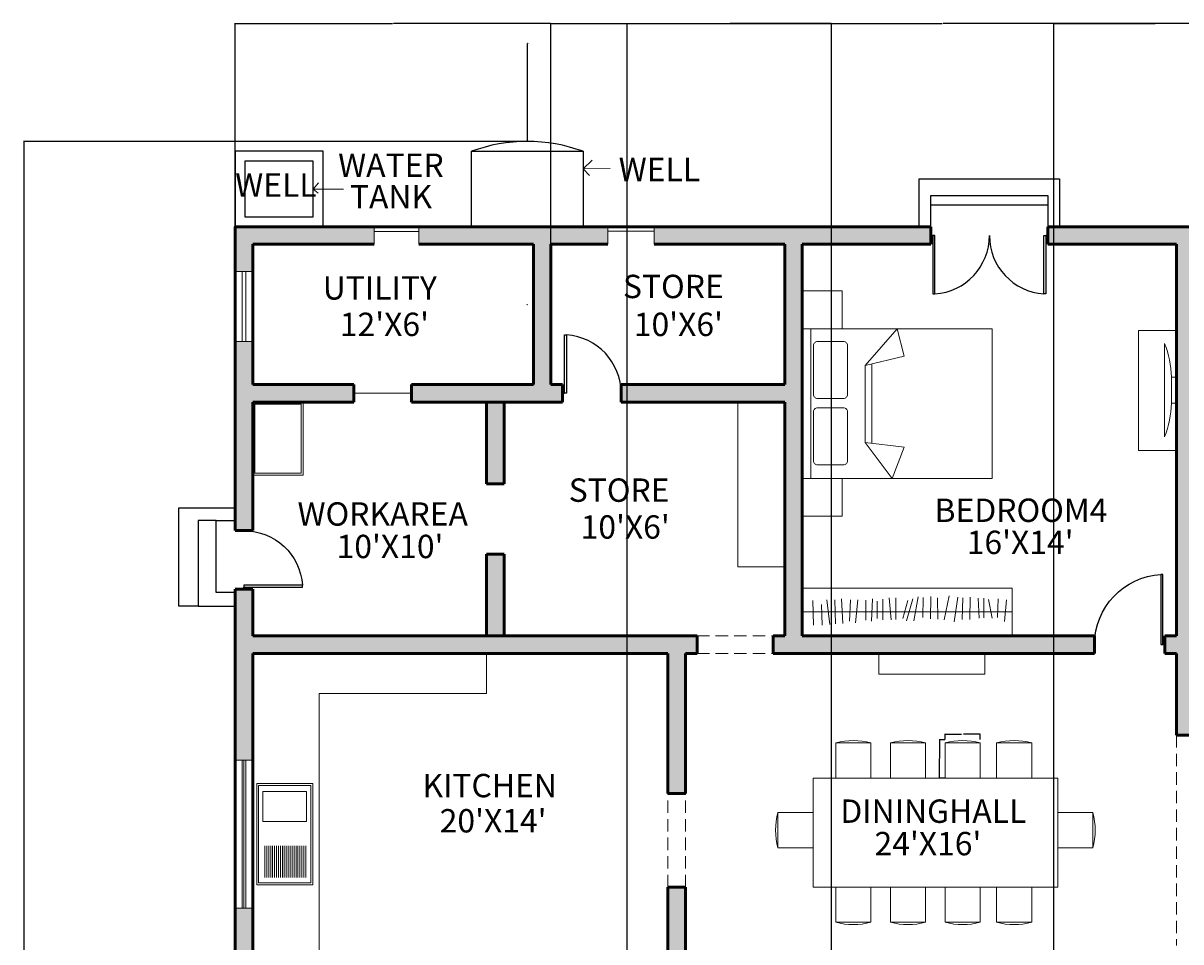
# Model space of a CAD drawing. Units: inches. Extents: x 2743 to 3669, y 1014 to 2282.
# Tile 4 of 5: x 2743 to 3337, y 1810 to 2282. Entities that reach past the tile are written whole.
import ezdxf

# ---------------------------------------------------------------- set-up
doc = ezdxf.new("R2010")
doc.units = ezdxf.units.IN
doc.linetypes.add('DASHED2', pattern=[9.525, 6.35, -3.175])
for name, color, linetype, lineweight in [('A-ANNO-DIMS', 2, 'Continuous', 18), ('A-ANNO-SYMB', 7, 'Continuous', 18), ('A-ANNO-TEXT', 4, 'Continuous', 18), ('A-AREA-IDEN', 4, 'Continuous', 18), ('A-DOOR', 211, 'Continuous', 25), ('A-EQPM', 51, 'Continuous', 18), ('A-FLOR-CASE', 51, 'Continuous', 18), ('A-FLOR-FIXT-PATT', 8, 'Continuous', 13), ('A-FLOR-STRS', 7, 'Continuous', 25), ('A-FURN', 111, 'Continuous', 18), ('A-GLAZ', 40, 'Continuous', 20), ('A-WALL', 7, 'Continuous', 50), ('A-WALL-OVHD', 8, 'DASHED2', 18), ('P-EQPM', 4, 'Continuous', 25)]:
    doc.layers.add(name, color=color, linetype=linetype, lineweight=lineweight)
doc.layers.add('A-FLOR-FIXT', color=11, linetype='Continuous', lineweight=18, true_color=0xee778f)
doc.layers.add('A-WALL-PATT', color=47, linetype='Continuous', lineweight=13, true_color=0x726c55)
doc.styles.get("Standard").update_dxf_attribs({"font": 'arial.ttf'})
doc.dimstyles.get("Standard").update_dxf_attribs({"dimtxt": 0.18, "dimasz": 0.18, "dimexe": 0.18, "dimexo": 0.0625, "dimgap": 0.09, "dimtad": 0, "dimtih": 1, "dimtoh": 1, "dimdec": 4, "dimzin": 0, "dimdsep": 46, "dimtxsty": 'Standard', "dimcen": 0.09, "dimadec": 0, "dimazin": 0, "dimtfac": 1, "dimtdec": 4, "dimtofl": 0, "dimtmove": 0, "dimatfit": 3, "dimfxl": 1, "dimtolj": 1, "dimtzin": 0, "dimarcsym": 0})

# ---------------------------------------------------------------- blocks, each defined once
blk = doc.blocks.new('DOOR-PAIR-60IN')
for p, q in [((0, 30), (1, 30)), ((1, 30), (1, 0)), ((2, 30), (1, 30)), ((2, 0), (2, 30)), ((58, 0), (58, 30)), ((58, 30), (59, 30)), ((60, 30), (59, 30)), ((59, 30), (59, 0)), ((1, 0), (2, 0)), ((59, 0), (58, 0))]:
    blk.add_line(p, q)
for centre, start, end in [((0, 29.93), 273.82241, 0.12746), ((60, 29.93), 179.99998, 266.1773)]:
    blk.add_arc(centre, 30, start, end)
blk = doc.blocks.new('DOOR-SINGLE-30IN')
for p, q in [((1, 0), (1, 30)), ((1, 30), (2, 30)), ((2, 30), (2, 0)), ((0, 0), (1, 0)), ((2, 0), (1, 0))]:
    blk.add_line(p, q)
blk.add_arc((0, 0.07), 30, 359.87254, 86.17759)
blk = doc.blocks.new('DOOR-SINGLE-36IN')
for p, q in [((1, 0), (1, 36)), ((1, 36), (2, 36)), ((2, 36), (2, 0)), ((0, 0), (1, 0)), ((2, 0), (1, 0))]:
    blk.add_line(p, q)
blk.add_arc((0, 0.06), 36, 359.91152, 86.81533)
blk = doc.blocks.new('WINDOW-36IN')
for p, q in [((9, 36), (0, 36)), ((3.5, 36), (3.5, 0)), ((5.5, 36), (5.5, 0)), ((9, 0), (0, 0))]:
    blk.add_line(p, q)
blk = doc.blocks.new('BED-DOUBLE')
for p, q in [((4.31, 76.75), (4.31, 0)), ((32.31, 57.96), (48.69, 76.75)), ((48.69, 76.75), (52.23, 62.72)), ((52.23, 62.72), (32.31, 57.96)), ((32.31, 18.34), (32.31, 57.96)), ((35.7, 17.95), (35.72, 58.78)), ((46.06, 0), (32.31, 18.34)), ((52.23, 16.05), (32.31, 18.34)), ((46.06, 0), (52.23, 16.05))]:
    blk.add_line(p, q)
blk.add_lwpolyline([(0, 76.75), (97.38, 76.75), (97.38, 0), (0, 0)], close=True)
for points in [[(7.76, 70.21), (21.16, 70.21, -0.414214), (23.16, 68.21), (23.16, 43, -0.414214), (21.16, 41), (7.76, 41, -0.414214), (5.76, 43), (5.76, 68.21, -0.414214)], [(7.76, 36.18), (21.16, 36.18, -0.414214), (23.16, 34.18), (23.16, 8.97, -0.414214), (21.16, 6.97), (7.76, 6.97, -0.414214), (5.76, 8.97), (5.76, 34.18, -0.414214)]]:
    blk.add_lwpolyline(points, format="xyb", close=True)
blk = doc.blocks.new('NIGHTSTAND')
blk.add_lwpolyline([(0, 0), (20.5, 0), (20.5, 19.45), (0, 19.45)], close=True)
blk = doc.blocks.new('CHAIR-DINING')
for p, q in [((0, 0), (0, 18)), ((0, 18), (18, 18)), ((18, 18), (18, 0))]:
    blk.add_line(p, q)
blk.add_arc((9, -14.1), 33.34, 74.33691, 105.66309)
blk = doc.blocks.new('*D22')
at = {"layer": 'A-ANNO-DIMS', "color": 0, "lineweight": -2, "transparency": 16777216}
for p, q in [((3216, 1913.74), (3212.93, 1913.74)), ((3213.11, 1913.56), (3213.11, 1904.1)), ((3213.11, 1894.27), (3213.11, 1903.73)), ((3216, 1894.09), (3212.93, 1894.09))]:
    blk.add_line(p, q, dxfattribs=at)
at = {"layer": 'A-ANNO-DIMS', "color": 0, "transparency": 16777216}
for points in [[(3213.08, 1913.56), (3213.14, 1913.56), (3213.11, 1913.74)], [(3213.08, 1894.27), (3213.14, 1894.27), (3213.11, 1894.09)]]:
    blk.add_solid(points, dxfattribs=at)
at = {"layer": 'Defpoints', "color": 0, "transparency": 16777216}
for p in [(3213.11, 1913.74), (3216.06, 1913.74), (3216.06, 1894.09)]:
    blk.add_point(p, dxfattribs=at)
at = {"layer": 'A-ANNO-DIMS', "color": 0, "transparency": 16777216, "insert": (3213.11, 1903.92), "char_height": 0.18, "attachment_point": 5}
blk.add_mtext('\\A1;CHAIR 20 TYP.', dxfattribs=at)
blk = doc.blocks.new('*D23')
at = {"layer": 'A-ANNO-DIMS', "color": 0, "lineweight": -2, "transparency": 16777216}
for p, q in [((3216.06, 1913.8), (3216.06, 1916.87)), ((3216.24, 1916.69), (3224.54, 1916.69)), ((3233.88, 1916.69), (3225.58, 1916.69)), ((3234.06, 1913.8), (3234.06, 1916.87))]:
    blk.add_line(p, q, dxfattribs=at)
at = {"layer": 'A-ANNO-DIMS', "color": 0, "transparency": 16777216}
for points in [[(3216.24, 1916.72), (3216.24, 1916.66), (3216.06, 1916.69)], [(3233.88, 1916.72), (3233.88, 1916.66), (3234.06, 1916.69)]]:
    blk.add_solid(points, dxfattribs=at)
at = {"layer": 'Defpoints', "color": 0, "transparency": 16777216}
for p in [(3216.06, 1913.74), (3234.06, 1916.69), (3234.06, 1913.74)]:
    blk.add_point(p, dxfattribs=at)
at = {"layer": 'A-ANNO-DIMS', "color": 0, "transparency": 16777216, "insert": (3225.06, 1916.69), "char_height": 0.18, "attachment_point": 5}
blk.add_mtext('\\A1;18 TYP.', dxfattribs=at)
blk = doc.blocks.new('*D62')
at = {"layer": 'A-ANNO-DIMS', "color": 0, "lineweight": -2, "transparency": 16777216}
for p, q in [((3608.38, 1899.55), (3608.38, 1014.41)), ((2803.91, 1765.52), (2803.91, 1014.41)), ((2804.09, 1014.59), (3205.75, 1014.59)), ((3608.2, 1014.59), (3206.54, 1014.59))]:
    blk.add_line(p, q, dxfattribs=at)
at = {"layer": 'A-ANNO-DIMS', "color": 0, "transparency": 16777216}
for points in [[(2804.09, 1014.62), (2804.09, 1014.56), (2803.91, 1014.59)], [(3608.2, 1014.62), (3608.2, 1014.56), (3608.38, 1014.59)]]:
    blk.add_solid(points, dxfattribs=at)
at = {"layer": 'Defpoints', "color": 0, "transparency": 16777216}
for p in [(3608.38, 1899.61), (2803.91, 1765.58), (3608.38, 1014.59)]:
    blk.add_point(p, dxfattribs=at)
at = {"layer": 'A-ANNO-DIMS', "color": 0, "transparency": 16777216, "insert": (3206.15, 1014.59), "char_height": 0.18, "attachment_point": 5}
blk.add_mtext('\\A1;804.5', dxfattribs=at)
blk = doc.blocks.new('*D63')
at = {"layer": 'A-ANNO-DIMS', "color": 0, "lineweight": -2, "transparency": 16777216}
for p, q in [((3001.57, 2220.87), (2743.18, 2220.87)), ((2743.36, 2220.69), (2743.36, 1648.19)), ((2743.36, 1075.32), (2743.36, 1647.82)), ((3214.73, 1075.14), (2743.18, 1075.14))]:
    blk.add_line(p, q, dxfattribs=at)
at = {"layer": 'A-ANNO-DIMS', "color": 0, "transparency": 16777216}
for points in [[(2743.33, 2220.69), (2743.39, 2220.69), (2743.36, 2220.87)], [(2743.33, 1075.32), (2743.39, 1075.32), (2743.36, 1075.14)]]:
    blk.add_solid(points, dxfattribs=at)
at = {"layer": 'Defpoints', "color": 0, "transparency": 16777216}
for p in [(2743.36, 2220.87), (3001.63, 2220.87), (3214.8, 1075.14)]:
    blk.add_point(p, dxfattribs=at)
at = {"layer": 'A-ANNO-DIMS', "color": 0, "transparency": 16777216, "insert": (2743.36, 1648.01), "char_height": 0.18, "attachment_point": 5}
blk.add_mtext('\\A1;1145.7', dxfattribs=at)
blk = doc.blocks.new('*D64')
at = {"layer": 'A-ANNO-DIMS', "color": 0, "lineweight": -2, "transparency": 16777216}
for p, q in [((2851.8, 2177.16), (2851.8, 2281.6)), ((2851.98, 2281.42), (2932.52, 2281.42)), ((3013.62, 2281.42), (2933.08, 2281.42)), ((3013.8, 2168.16), (3013.8, 2281.6))]:
    blk.add_line(p, q, dxfattribs=at)
at = {"layer": 'A-ANNO-DIMS', "color": 0, "transparency": 16777216}
for points in [[(2851.98, 2281.45), (2851.98, 2281.39), (2851.8, 2281.42)], [(3013.62, 2281.45), (3013.62, 2281.39), (3013.8, 2281.42)]]:
    blk.add_solid(points, dxfattribs=at)
at = {"layer": 'Defpoints', "color": 0, "transparency": 16777216}
for p in [(3013.8, 2281.42), (2851.8, 2177.09), (3013.8, 2168.09)]:
    blk.add_point(p, dxfattribs=at)
at = {"layer": 'A-ANNO-DIMS', "color": 0, "transparency": 16777216, "insert": (2932.8, 2281.42), "char_height": 0.18, "attachment_point": 5}
blk.add_mtext('\\A1;162', dxfattribs=at)
blk = doc.blocks.new('*D65')
at = {"layer": 'A-ANNO-DIMS', "color": 0, "lineweight": -2, "transparency": 16777216}
for p, q in [((3013.8, 2168.16), (3013.8, 2281.6)), ((3013.98, 2281.42), (3214.5, 2281.42)), ((3415.62, 2281.42), (3215.09, 2281.42)), ((3415.8, 2168.16), (3415.8, 2281.6))]:
    blk.add_line(p, q, dxfattribs=at)
at = {"layer": 'A-ANNO-DIMS', "color": 0, "transparency": 16777216}
for points in [[(3013.98, 2281.45), (3013.98, 2281.39), (3013.8, 2281.42)], [(3415.62, 2281.45), (3415.62, 2281.39), (3415.8, 2281.42)]]:
    blk.add_solid(points, dxfattribs=at)
at = {"layer": 'Defpoints', "color": 0, "transparency": 16777216}
for p in [(3415.8, 2281.42), (3013.8, 2168.09), (3415.8, 2168.09)]:
    blk.add_point(p, dxfattribs=at)
at = {"layer": 'A-ANNO-DIMS', "color": 0, "transparency": 16777216, "insert": (3214.8, 2281.42), "char_height": 0.18, "attachment_point": 5}
blk.add_mtext('\\A1;402', dxfattribs=at)
blk = doc.blocks.new('*D76')
at = {"layer": 'A-ANNO-DIMS', "color": 0, "lineweight": -2, "transparency": 16777216}
for p, q in [((3052.84, 1130.9), (3052.84, 2281.6)), ((3053.02, 2281.42), (3104.86, 2281.42)), ((3157.62, 2281.42), (3105.77, 2281.42)), ((3157.8, 1130.9), (3157.8, 2281.6))]:
    blk.add_line(p, q, dxfattribs=at)
at = {"layer": 'A-ANNO-DIMS', "color": 0, "transparency": 16777216}
for points in [[(3053.02, 2281.45), (3053.02, 2281.39), (3052.84, 2281.42)], [(3157.62, 2281.45), (3157.62, 2281.39), (3157.8, 2281.42)]]:
    blk.add_solid(points, dxfattribs=at)
at = {"layer": 'Defpoints', "color": 0, "transparency": 16777216}
for p in [(3157.8, 2281.42), (3052.84, 1130.83), (3157.8, 1130.83)]:
    blk.add_point(p, dxfattribs=at)
at = {"layer": 'A-ANNO-DIMS', "color": 0, "transparency": 16777216, "insert": (3105.32, 2281.42), "char_height": 0.18, "attachment_point": 5}
blk.add_mtext('\\A1;104.95', dxfattribs=at)
blk = doc.blocks.new('*D77')
at = {"layer": 'A-ANNO-DIMS', "color": 0, "lineweight": -2, "transparency": 16777216}
for p, q in [((3157.8, 1130.9), (3157.8, 2281.6)), ((3157.98, 2281.42), (3214.52, 2281.42)), ((3271.62, 2281.42), (3215.08, 2281.42)), ((3271.8, 1130.9), (3271.8, 2281.6))]:
    blk.add_line(p, q, dxfattribs=at)
at = {"layer": 'A-ANNO-DIMS', "color": 0, "transparency": 16777216}
for points in [[(3157.98, 2281.45), (3157.98, 2281.39), (3157.8, 2281.42)], [(3271.62, 2281.45), (3271.62, 2281.39), (3271.8, 2281.42)]]:
    blk.add_solid(points, dxfattribs=at)
at = {"layer": 'Defpoints', "color": 0, "transparency": 16777216}
for p in [(3271.8, 2281.42), (3157.8, 1130.83), (3271.8, 1130.83)]:
    blk.add_point(p, dxfattribs=at)
at = {"layer": 'A-ANNO-DIMS', "color": 0, "transparency": 16777216, "insert": (3214.8, 2281.42), "char_height": 0.18, "attachment_point": 5}
blk.add_mtext('\\A1;114', dxfattribs=at)
blk = doc.blocks.new('*D78')
at = {"layer": 'A-ANNO-DIMS', "color": 0, "lineweight": -2, "transparency": 16777216}
for p, q in [((3271.8, 1130.9), (3271.8, 2281.6)), ((3271.98, 2281.42), (3323.82, 2281.42)), ((3376.57, 2281.42), (3324.73, 2281.42)), ((3376.75, 1130.9), (3376.75, 2281.6))]:
    blk.add_line(p, q, dxfattribs=at)
at = {"layer": 'A-ANNO-DIMS', "color": 0, "transparency": 16777216}
for points in [[(3271.98, 2281.45), (3271.98, 2281.39), (3271.8, 2281.42)], [(3376.57, 2281.45), (3376.57, 2281.39), (3376.75, 2281.42)]]:
    blk.add_solid(points, dxfattribs=at)
at = {"layer": 'Defpoints', "color": 0, "transparency": 16777216}
for p in [(3376.75, 2281.42), (3271.8, 1130.83), (3376.75, 1130.83)]:
    blk.add_point(p, dxfattribs=at)
at = {"layer": 'A-ANNO-DIMS', "color": 0, "transparency": 16777216, "insert": (3324.27, 2281.42), "char_height": 0.18, "attachment_point": 5}
blk.add_mtext('\\A1;104.95', dxfattribs=at)
blk = doc.blocks.new('*D79')
at = {"layer": 'A-ANNO-DIMS', "color": 0, "lineweight": -2, "transparency": 16777216}
for p, q in [((3001.81, 2271.08), (3001.63, 2271.08)), ((3001.63, 2271.08), (3001.63, 2221.05)), ((3001.54, 2137.19), (3001.72, 2137.19)), ((3001.63, 2137.1), (3001.63, 2137.28))]:
    blk.add_line(p, q, dxfattribs=at)
at = {"layer": 'A-ANNO-DIMS', "color": 0, "transparency": 16777216}
blk.add_solid([(3001.6, 2221.05), (3001.66, 2221.05), (3001.63, 2220.87)], dxfattribs=at)
at = {"layer": 'Defpoints', "color": 0, "transparency": 16777216}
for p in [(3001.63, 2220.87), (3001.63, 2137.19)]:
    blk.add_point(p, dxfattribs=at)
at = {"layer": 'A-ANNO-DIMS', "color": 0, "transparency": 16777216, "insert": (3002.29, 2271.08), "char_height": 0.18, "attachment_point": 5}
blk.add_mtext('\\A1;R83.68', dxfattribs=at)

msp = doc.modelspace()

# ---------------------------------------------------------------- hatches: boundary and pattern name
at = {"layer": 'A-FLOR-FIXT-PATT'}
h = msp.add_hatch(dxfattribs=at)
h.set_pattern_fill('ANSI31', color=256, scale=0.3149606, angle=45, style=0)
h.paths.add_polyline_path([(2866.394, 1843.128), (2888.374, 1843.128), (2888.374, 1859.253), (2866.394, 1859.253)])
at = {"layer": 'A-WALL-PATT'}
h = msp.add_hatch(color=256, dxfattribs=at)
h.dxf.hatch_style = 1
h.paths.add_polyline_path([(2923.052, 2168.094), (2923.052, 2177.094), (2851.796, 2177.094), (2851.796, 2154.151), (2860.796, 2154.151), (2860.796, 2168.094)])
h = msp.add_hatch(color=256, dxfattribs=at)
h.dxf.hatch_style = 1
h.paths.add_polyline_path([(3004.796, 2168.094), (3004.796, 2096.094), (2942.31, 2096.094), (2942.31, 2087.094), (3019.796, 2087.094), (3019.796, 2096.094), (3013.796, 2096.094), (3013.796, 2168.094), (3043.074, 2168.094), (3043.074, 2177.094), (2946.082, 2177.094), (2946.082, 2168.094)])
h = msp.add_hatch(color=256, dxfattribs=at)
h.dxf.hatch_style = 1
h.paths.add_polyline_path([(3066.832, 2177.094), (3066.832, 2168.094), (3133.796, 2168.094), (3133.796, 2096.094), (3049.796, 2096.094), (3049.796, 2087.094), (3133.796, 2087.094), (3133.796, 2002.521), (3133.796, 1967.094), (3127.796, 1967.094), (3127.796, 1958.094), (3292.796, 1958.094), (3292.796, 1967.094), (3142.796, 1967.094), (3142.796, 1991.577), (3142.796, 2168.094), (3208.796, 2168.094), (3208.796, 2177.094), (3202.796, 2177.094)])
h = msp.add_hatch(color=256, dxfattribs=at)
h.dxf.hatch_style = 1
h.paths.add_polyline_path([(3334.796, 2168.094), (3334.796, 1967.094), (3328.796, 1967.094), (3328.796, 1958.094), (3334.796, 1958.094), (3334.796, 1916.094), (3343.796, 1916.094), (3343.796, 1958.094), (3349.796, 1958.094), (3349.796, 1967.094), (3343.796, 1967.094), (3343.796, 2030.094), (3379.796, 2030.094), (3379.796, 2039.094), (3343.796, 2039.094), (3343.796, 2087.094), (3367.124, 2087.094), (3367.124, 2096.094), (3343.796, 2096.094), (3343.796, 2168.094), (3363.161, 2168.094), (3363.161, 2177.094), (3268.796, 2177.094), (3268.796, 2168.094)])
h = msp.add_hatch(color=256, dxfattribs=at)
h.dxf.hatch_style = 1
h.paths.add_polyline_path([(2886.631, 2087.094), (2912.654, 2087.094), (2912.654, 2096.094), (2860.796, 2096.094), (2860.796, 2118.151), (2851.796, 2118.151), (2851.796, 2021.094), (2860.796, 2021.094), (2860.796, 2087.094)])
h = msp.add_hatch(color=256, dxfattribs=at)
h.dxf.hatch_style = 1
h.paths.add_polyline_path([(2989.796, 2087.094), (2980.796, 2087.094), (2980.796, 2045.094), (2989.796, 2045.094)])
h = msp.add_hatch(color=256, dxfattribs=at)
h.dxf.hatch_style = 1
h.paths.add_polyline_path([(2989.796, 2009.094), (2980.796, 2009.094), (2980.796, 1967.094), (2989.796, 1967.094)])
h = msp.add_hatch(color=256, dxfattribs=at)
h.dxf.hatch_style = 1
h.paths.add_polyline_path([(2860.796, 1967.094), (2860.796, 1991.094), (2851.796, 1991.094), (2851.796, 1903.347), (2860.796, 1903.347), (2860.796, 1958.094), (3073.796, 1958.094), (3073.796, 1886.094), (3082.796, 1886.094), (3082.796, 1958.094), (3088.796, 1958.094), (3088.796, 1967.094)])
h = msp.add_hatch(color=256, dxfattribs=at)
h.dxf.hatch_style = 1
h.paths.add_polyline_path([(3082.796, 1838.094), (3073.796, 1838.094), (3073.796, 1766.094), (3021.39, 1766.094), (2860.796, 1766.094), (2860.796, 1827.347), (2851.796, 1827.347), (2851.796, 1745.094), (2860.796, 1745.094), (2860.796, 1757.094), (3004.796, 1757.094), (3004.796, 1672.878), (3013.796, 1672.878), (3013.796, 1757.094), (3105.339, 1757.094), (3105.339, 1766.094), (3082.796, 1766.094)])

# ---------------------------------------------------------------- linework, layer by layer
at = {"layer": 'A-ANNO-SYMB'}
for p, q in [((3030.296, 2206.805), (3034.892, 2211.217)), ((3030.296, 2206.805), (3044.277, 2206.915)), ((3030.296, 2206.805), (3030.296, 2206.805)), ((3030.296, 2206.805), (3033.61, 2203.354)), ((2891.879, 2196.451), (2894.463, 2199.563)), ((2891.879, 2199.053), (2891.879, 2199.053)), ((2891.879, 2197.699), (2891.879, 2197.699)), ((2896.879, 2196.451), (2891.879, 2196.451)), ((2891.879, 2196.451), (2894.347, 2194.402)), ((2896.879, 2196.451), (2907.327, 2196.451))]:
    msp.add_line(p, q, dxfattribs=at)
at = {"layer": 'A-EQPM'}
for p, q in [((3315.266, 2062.302), (3315.266, 2123.901)), ((3315.266, 2123.901), (3334.796, 2123.901)), ((3334.796, 2123.901), (3334.796, 2062.302)), ((3328.688, 2117.192), (3328.688, 2069.302)), ((3334.796, 2099.943), (3332.16, 2099.943)), ((3332.16, 2099.943), (3332.16, 2086.558)), ((3334.796, 2086.558), (3334.796, 2099.943)), ((3332.16, 2086.558), (3334.796, 2086.558)), ((3334.796, 2062.302), (3315.266, 2062.302))]:
    msp.add_line(p, q, dxfattribs=at)
for centre, radius, start, end in [((3280.052, 2098.429), 52.13, 1.664643, 21.096452), ((3280.127, 2088.05), 52.054, 338.889928, 358.357911)]:
    msp.add_arc(centre, radius, start, end, dxfattribs=at)
at = {"layer": 'A-FLOR-CASE'}
for p, q in [((3148.137, 1985.224), (3148.495, 1972.526)), ((3155.297, 1985.582), (3156.908, 1972.883)), ((3159.414, 1985.582), (3159.772, 1973.241)), ((3162.815, 1986.118), (3163.58, 1973.351)), ((3167.469, 1985.582), (3166.932, 1974.672)), ((3171.228, 1985.582), (3170.154, 1973.778)), ((3175.346, 1985.403), (3175.346, 1975.208)), ((3178.747, 1986.118), (3178.21, 1974.672)), ((3181.253, 1984.866), (3181.253, 1975.924)), ((3184.117, 1985.939), (3184.117, 1975.387)), ((3187.339, 1986.655), (3188.413, 1975.387)), ((3190.74, 1986.655), (3190.74, 1975.566)), ((3197.005, 1985.224), (3194.32, 1975.924)), ((3199.511, 1986.118), (3196.254, 1974.837)), ((3202.196, 1987.191), (3200.048, 1974.837)), ((3204.749, 1986.747), (3204.702, 1976.46)), ((3208.819, 1987.37), (3208.64, 1975.745)), ((3212.22, 1986.655), (3212.404, 1975.687)), ((3218.128, 1987.549), (3215.622, 1975.387)), ((3222.603, 1987.013), (3220.634, 1974.314)), ((3225.109, 1986.655), (3224.751, 1975.566)), ((3228.868, 1987.013), (3228.689, 1975.566)), ((3232.985, 1986.476), (3233.522, 1976.103)), ((3235.849, 1986.476), (3235.849, 1976.281)), ((3238.355, 1985.761), (3240.145, 1976.103)), ((3243.367, 1986.118), (3243.009, 1976.46)), ((3247.484, 1985.582), (3246.589, 1974.493)), ((3142.796, 1979.335), (3250.483, 1979.335)), ((3152.97, 1972.526), (3152.671, 1983.14)), ((2980.796, 1958.094), (2980.796, 1937.562)), ((2980.796, 1937.562), (2894.795, 1937.562)), ((2894.795, 1937.562), (2894.795, 1798.541))]:
    msp.add_line(p, q, dxfattribs=at)
for points in [[(3133.796, 2087.094), (3109.755, 2087.094), (3109.755, 2002.521), (3133.796, 2002.521)], [(3142.796, 1967.094), (3250.483, 1967.094), (3250.483, 1991.577), (3142.796, 1991.577)], [(3182.11, 1958.094), (3236.392, 1958.094), (3236.392, 1947.343), (3182.11, 1947.343)]]:
    msp.add_lwpolyline(points, close=True, dxfattribs=at)
at = {"layer": 'A-FLOR-FIXT'}
for points in [[(2860.796, 2087.094), (2886.631, 2087.094), (2886.631, 2049.618), (2860.796, 2049.618)], [(2861.796, 2086.094), (2885.631, 2086.094), (2885.631, 2050.618), (2861.796, 2050.618)], [(2862.81, 1891.213), (2891.559, 1891.213), (2891.559, 1839.294), (2862.81, 1839.294)], [(2863.81, 1890.213), (2890.559, 1890.213), (2890.559, 1840.294), (2863.81, 1840.294)], [(2865.916, 1887.16), (2888.422, 1887.16), (2888.422, 1871.846), (2865.916, 1871.846)]]:
    msp.add_lwpolyline(points, close=True, dxfattribs=at)
at = {"layer": 'A-FLOR-STRS'}
for p, q in [((3202.796, 2177.094), (3202.796, 2201.655)), ((3202.796, 2201.655), (3274.796, 2201.655)), ((3274.796, 2201.655), (3274.796, 2177.094)), ((3208.796, 2177.094), (3208.796, 2193.212)), ((3208.796, 2193.212), (3268.796, 2193.212)), ((3268.796, 2193.212), (3268.796, 2177.094)), ((3208.796, 2188.298), (3268.796, 2188.298)), ((3208.796, 2177.094), (3202.796, 2177.094)), ((2822.946, 1982.302), (2822.946, 2032.795)), ((2822.946, 2032.795), (2851.796, 2032.795)), ((2842.021, 2026.297), (2832.837, 2026.297)), ((2832.837, 2026.297), (2832.837, 1982.302)), ((2842.021, 1989.358), (2842.021, 2026.297)), ((2842.021, 2026.297), (2851.796, 2026.297)), ((2851.796, 1989.358), (2842.021, 1989.358)), ((2832.837, 1982.302), (2822.946, 1982.302)), ((2832.837, 1982.302), (2851.796, 1982.302))]:
    msp.add_line(p, q, dxfattribs=at)
at = {"layer": 'A-FURN'}
msp.add_lwpolyline([(3148.283, 1894.091), (3273.845, 1894.091), (3273.845, 1838.091), (3148.283, 1838.091)], close=True, dxfattribs=at)
at = {"layer": 'A-GLAZ'}
for p, q in [((2923.052, 2177.094), (2923.052, 2168.094)), ((2923.052, 2174.572), (2946.082, 2174.572)), ((2946.082, 2177.094), (2946.082, 2168.094)), ((3043.074, 2177.094), (3043.074, 2168.094)), ((3043.074, 2174.86), (3066.832, 2174.86)), ((3066.832, 2177.094), (3066.832, 2168.094)), ((2912.654, 2091.594), (2942.31, 2091.594)), ((2851.796, 1903.347), (2860.796, 1903.347)), ((2855.296, 1903.347), (2855.296, 1827.347)), ((2856.296, 1903.347), (2856.296, 1827.347)), ((2857.296, 1903.347), (2857.296, 1827.347)), ((2851.796, 1827.347), (2860.796, 1827.347))]:
    msp.add_line(p, q, dxfattribs=at)
at = {"layer": 'A-WALL'}
for p, q in [((3208.796, 2168.094), (3208.796, 2177.094)), ((3268.796, 2168.094), (3268.796, 2177.094)), ((2860.796, 2168.094), (2923.052, 2168.094)), ((2860.796, 2096.094), (2860.796, 2168.094)), ((2946.082, 2168.094), (3004.796, 2168.094)), ((3004.796, 2096.094), (3004.796, 2168.094)), ((3013.796, 2096.094), (3013.796, 2168.094)), ((3013.796, 2168.094), (3043.074, 2168.094)), ((3066.832, 2168.094), (3133.796, 2168.094)), ((3133.796, 2096.094), (3133.796, 2168.094)), ((3142.796, 1967.094), (3142.796, 2168.094)), ((3142.796, 2168.094), (3208.796, 2168.094)), ((3268.796, 2168.094), (3334.796, 2168.094)), ((3334.796, 1967.094), (3334.796, 2168.094)), ((2860.796, 2096.094), (2912.654, 2096.094)), ((2912.654, 2087.094), (2912.654, 2096.094)), ((2942.31, 2087.094), (2942.31, 2096.094)), ((2942.31, 2096.094), (3004.796, 2096.094)), ((3013.796, 2096.094), (3019.796, 2096.094)), ((3019.796, 2087.094), (3019.796, 2096.094)), ((3049.796, 2087.094), (3049.796, 2096.094)), ((3049.796, 2096.094), (3133.796, 2096.094)), ((2860.796, 2087.094), (2912.654, 2087.094)), ((2860.796, 2021.094), (2860.796, 2087.094)), ((2942.31, 2087.094), (3019.796, 2087.094)), ((2980.796, 2045.094), (2980.796, 2087.094)), ((2989.796, 2045.094), (2989.796, 2087.094)), ((3049.796, 2087.094), (3133.796, 2087.094)), ((3133.796, 1967.094), (3133.796, 2087.094)), ((2980.796, 2045.094), (2989.796, 2045.094)), ((2860.796, 2021.094), (2851.796, 2021.094)), ((2980.796, 1967.094), (2980.796, 2009.094)), ((2980.796, 2009.094), (2989.796, 2009.094)), ((2989.796, 1967.094), (2989.796, 2009.094)), ((2860.796, 1991.094), (2851.796, 1991.094)), ((2860.796, 1967.094), (2860.796, 1991.094)), ((2860.796, 1967.094), (3088.796, 1967.094)), ((3088.796, 1958.094), (3088.796, 1967.094)), ((3127.796, 1967.094), (3127.796, 1958.094)), ((3127.796, 1967.094), (3133.796, 1967.094)), ((3142.796, 1967.094), (3292.796, 1967.094)), ((3292.796, 1967.094), (3292.796, 1958.094)), ((3328.796, 1967.094), (3328.796, 1958.094)), ((3328.796, 1967.094), (3334.796, 1967.094)), ((2860.796, 1958.094), (3073.796, 1958.094)), ((2860.796, 1766.094), (2860.796, 1958.094)), ((3073.796, 1886.094), (3073.796, 1958.094)), ((3082.796, 1886.094), (3082.796, 1958.094)), ((3082.796, 1958.094), (3088.796, 1958.094)), ((3127.796, 1958.094), (3292.796, 1958.094)), ((3328.796, 1958.094), (3334.796, 1958.094)), ((3334.796, 1916.094), (3334.796, 1958.094)), ((3334.796, 1916.094), (3343.796, 1916.094)), ((3073.796, 1886.094), (3082.796, 1886.094)), ((3073.796, 1766.094), (3073.796, 1838.094)), ((3073.796, 1838.094), (3082.796, 1838.094)), ((3082.796, 1766.094), (3082.796, 1838.094))]:
    msp.add_line(p, q, dxfattribs=at)
for points in [[(2851.796, 2021.094), (2851.796, 2177.094), (3208.796, 2177.094)], [(3268.796, 2177.094), (3577.796, 2177.094), (3577.796, 1886.608)], [(2851.796, 1745.094), (2851.796, 1991.094)]]:
    msp.add_lwpolyline(points, dxfattribs=at)
at = {"layer": 'A-WALL-OVHD'}
for p, q in [((3088.796, 1967.094), (3127.796, 1967.094)), ((3088.796, 1958.094), (3127.796, 1958.094)), ((3334.796, 1916.094), (3334.796, 1808.094)), ((3073.796, 1838.094), (3073.796, 1886.094)), ((3082.796, 1838.094), (3082.796, 1886.094))]:
    msp.add_line(p, q, dxfattribs=at)
at = {"layer": 'P-EQPM'}
for points in [[(2851.796, 2177.094), (2896.879, 2177.094), (2896.879, 2215.808), (2851.796, 2215.808)], [(3030.296, 2177.094), (2972.961, 2177.094), (2972.961, 2215.808), (3030.296, 2215.808)], [(2856.796, 2182.094), (2891.879, 2182.094), (2891.879, 2210.808), (2856.796, 2210.808)]]:
    msp.add_lwpolyline(points, close=True, dxfattribs=at)
msp.add_arc((3001.629, 2137.188), 83.683, 69.966052, 110.033948, dxfattribs=at)

# ---------------------------------------------------------------- block references
at = {"layer": 'A-DOOR'}
for name, p in [('DOOR-PAIR-60IN', (3208.796, 2142.594)), ('DOOR-SINGLE-30IN', (3019.796, 2091.594))]:
    msp.add_blockref(name, p, dxfattribs=at)
at = {"layer": 'A-DOOR', "extrusion": (0, 0, -1), "zscale": -1, "rotation": 89.99999999999834}
msp.add_blockref('DOOR-SINGLE-30IN', (-2856.296, 1991.094), dxfattribs=at)
at = {"layer": 'A-DOOR', "extrusion": (0, 0, -1), "zscale": -1}
msp.add_blockref('DOOR-SINGLE-36IN', (-3328.797, 1962.594), dxfattribs=at)
at = {"layer": 'A-FURN'}
for name, p in [('NIGHTSTAND', (3142.796, 2124.692)), ('BED-DOUBLE', (3142.796, 2047.943)), ('NIGHTSTAND', (3142.796, 2028.495)), ('CHAIR-DINING', (3159.95, 1894.091)), ('CHAIR-DINING', (3188.013, 1894.091)), ('CHAIR-DINING', (3216.061, 1894.091)), ('CHAIR-DINING', (3242.487, 1894.091))]:
    msp.add_blockref(name, p, dxfattribs=at)
for p, rotation in [((3148.282, 1858.333), 90.00000000000055), ((3273.845, 1876.333), 269.9999999999984), ((3177.95, 1838.09), 180), ((3206.013, 1838.09), 180), ((3234.061, 1838.09), 180), ((3260.487, 1838.09), 180)]:
    msp.add_blockref('CHAIR-DINING', p, dxfattribs=dict(at, rotation=rotation))
at = {"layer": 'A-GLAZ'}
msp.add_blockref('WINDOW-36IN', (2851.796, 2118.151), dxfattribs=at)

# ---------------------------------------------------------------- texts
at = {"layer": 'A-ANNO-TEXT'}
for tag, p in [('WATER', (2904.613, 2202.671)), ('WELL', (3048.572, 2200.475)), ('WELL', (2851.796, 2192.515)), ('TANK', (2910.657, 2186.476))]:
    msp.add_attdef(tag, p, '', height=12, dxfattribs=at)
at = {"layer": 'A-AREA-IDEN'}
for tag, p in [('UTILITY', (2896.716, 2139.711)), ('STORE', (3050.755, 2140.44)), ("12'X6'", (2905.483, 2120.975)), ("10'X6'", (3056.321, 2120.975)), ('STORE', (3022.925, 2035.889)), ('BEDROOM4', (3210.641, 2025.552)), ('WORKAREA', (2883.775, 2023.654)), ("10'X6'", (3029.048, 2016.981)), ("16'X14'", (3227.148, 2009.059)), ("10'X10'", (2903.813, 2006.97)), ('KITCHEN', (2947.854, 1884.228)), ('DININGHALL', (3162.287, 1871.098)), ("20'X14'", (2956.717, 1866.164)), ("24'X16'", (3179.849, 1854.439))]:
    msp.add_attdef(tag, p, '', height=12, dxfattribs=at)

# ---------------------------------------------------------------- dimensions: what is measured, and where the dimension line sits
at = {"layer": 'A-ANNO-DIMS'}
for base, p1, p2, override, picture, middle in [((3013.796, 2281.421), (2851.796, 2177.094), (3013.796, 2168.094), {"dimdec": 0, "dimlfac": 1, "dimrnd": 0, "dimzin": 0, "dimdsep": 46, "dimlunit": 2}, '*D64', (2932.796, 2281.421)), ((3415.796, 2281.421), (3013.796, 2168.094), (3415.796, 2168.094), {"dimdec": 0, "dimlfac": 1, "dimrnd": 0, "dimzin": 0, "dimdsep": 46, "dimlunit": 2}, '*D65', (3214.796, 2281.421)), ((3157.796, 2281.421), (3052.842, 1130.835), (3157.796, 1130.835), {"dimdec": 2, "dimlfac": 1, "dimrnd": 0, "dimzin": 0, "dimdsep": 46, "dimlunit": 2}, '*D76', (3105.319, 2281.421)), ((3271.796, 2281.421), (3157.796, 1130.835), (3271.796, 1130.835), {"dimdec": 0, "dimlfac": 1, "dimrnd": 0, "dimzin": 0, "dimdsep": 46, "dimlunit": 2}, '*D77', (3214.796, 2281.421)), ((3376.7513, 2281.4212), (3271.7965, 1130.8347), (3376.7513, 1130.8347), {"dimdec": 2, "dimlfac": 1, "dimrnd": 0, "dimzin": 0, "dimdsep": 46, "dimlunit": 2}, '*D78', (3324.2739, 2281.4212)), ((3608.383, 1014.589), (2803.91, 1765.581), (3608.383, 1899.608), {"dimdec": 1, "dimlfac": 1, "dimrnd": 0, "dimzin": 0, "dimdsep": 46, "dimlunit": 2}, '*D62', (3206.146, 1014.589))]:
    dim = msp.add_linear_dim(base=base, p1=p1, p2=p2, dimstyle='Standard', override=override, dxfattribs=at)
    dim.commit()
    dim.dimension.update_dxf_attribs({"geometry": picture, "text_midpoint": middle})
dim = msp.add_radius_dim(center=(3001.629, 2137.188), mpoint=(3001.629, 2220.871), dimstyle='Standard', override={"dimdec": 2, "dimlfac": 1, "dimrnd": 0, "dimzin": 0, "dimdsep": 46, "dimlunit": 2}, dxfattribs=at)
dim.commit()
dim.dimension.update_dxf_attribs({"geometry": '*D79', "text_midpoint": (3002.289, 2271.081), "dimtype": 164})
dim = msp.add_linear_dim(base=(2743.36, 2220.871), p1=(3214.796, 1075.139), p2=(3001.629, 2220.871), angle=90, dimstyle='Standard', override={"dimdec": 1, "dimlfac": 1, "dimrnd": 0, "dimzin": 0, "dimdsep": 46, "dimlunit": 2}, dxfattribs=at)
dim.commit()
dim.dimension.update_dxf_attribs({"geometry": '*D63', "text_midpoint": (2743.36, 1648.005)})
dim = msp.add_linear_dim(base=(3213.114, 1913.741), p1=(3216.061, 1894.091), p2=(3216.061, 1913.741), angle=90, text='CHAIR <> TYP.', dimstyle='Standard', override={"dimdec": 0, "dimlfac": 1, "dimrnd": 0, "dimzin": 0, "dimdsep": 46, "dimlunit": 2}, dxfattribs=at)
dim.commit()
dim.dimension.update_dxf_attribs({"geometry": '*D22', "text_midpoint": (3213.114, 1903.916)})
dim = msp.add_linear_dim(base=(3234.061, 1916.689), p1=(3216.061, 1913.741), p2=(3234.061, 1913.741), text='<> TYP.', dimstyle='Standard', override={"dimdec": 0, "dimlfac": 1, "dimrnd": 0, "dimzin": 0, "dimdsep": 46, "dimlunit": 2}, dxfattribs=at)
dim.commit()
dim.dimension.update_dxf_attribs({"geometry": '*D23', "text_midpoint": (3225.061, 1916.689)})

doc.saveas('drawing.dxf')
